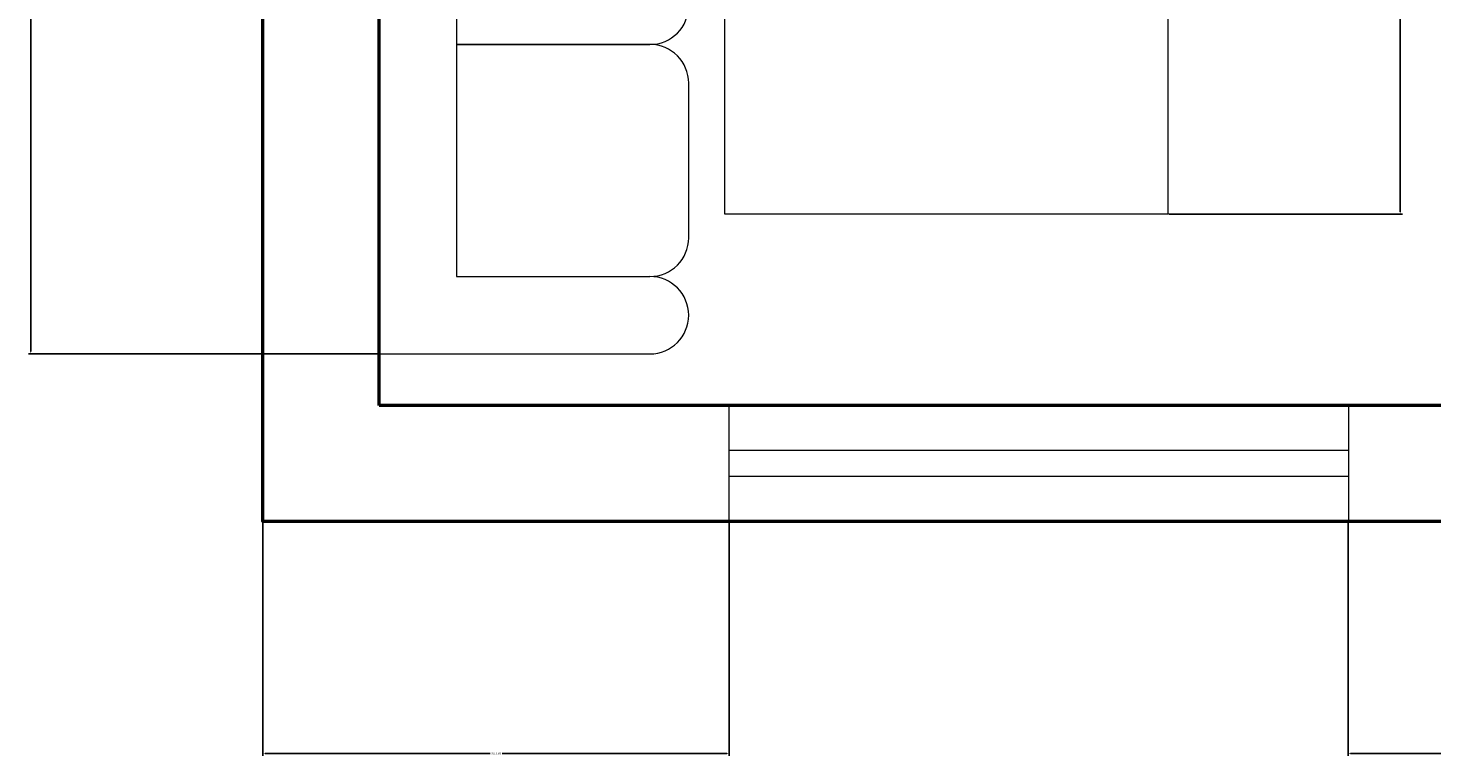
# Model space of a CAD drawing. Units: inches. Extents: x 2621 to 2849, y 2066 to 2463.
# Tile 1 of 28: x 2621 to 2729, y 2066 to 2123. Entities that reach past the tile are written whole.
import ezdxf

# ---------------------------------------------------------------- set-up
doc = ezdxf.new("R2010")
doc.units = ezdxf.units.IN
for name, color, linetype, lineweight in [('A-ANNO-DIMS', 2, 'Continuous', 18), ('A-FURN', 8, 'Continuous', 18), ('A-GLAZ', 4, 'Continuous', 18), ('A-WALL', 7, 'Continuous', 50)]:
    doc.layers.add(name, color=color, linetype=linetype, lineweight=lineweight)
doc.styles.get("Standard").update_dxf_attribs({"font": 'arial.ttf'})
doc.dimstyles.get("Standard").update_dxf_attribs({"dimtxt": 0.18, "dimasz": 0.18, "dimexe": 0.18, "dimexo": 0.0625, "dimgap": 0.09, "dimtad": 0, "dimtih": 1, "dimtoh": 1, "dimdec": 4, "dimzin": 0, "dimdsep": 46, "dimtxsty": 'Standard', "dimcen": 0.09, "dimadec": 0, "dimazin": 0, "dimtfac": 1, "dimtdec": 4, "dimtofl": 0, "dimtmove": 0, "dimatfit": 3, "dimfxl": 1, "dimtolj": 1, "dimtzin": 0, "dimarcsym": 0})

# ---------------------------------------------------------------- blocks, each defined once
blk = doc.blocks.new('WIN-48IN')
for p, q in [((0, 5.5), (48, 5.5)), ((0, 3.5), (48, 3.5))]:
    blk.add_line(p, q)
for points in [[(0, 0), (0, 9)], [(48, 9), (48, 0)]]:
    blk.add_lwpolyline(points)
blk = doc.blocks.new('*D40')
at = {"layer": 'A-ANNO-DIMS', "color": 0, "lineweight": -2, "transparency": 16777216}
for p, q in [((2638.87, 2084.31), (2638.87, 2066.19)), ((2675, 2084.31), (2675, 2066.19)), ((2639.05, 2066.37), (2656.47, 2066.37)), ((2674.82, 2066.37), (2657.4, 2066.37))]:
    blk.add_line(p, q, dxfattribs=at)
at = {"layer": 'A-ANNO-DIMS', "color": 0, "transparency": 16777216}
for points in [[(2639.05, 2066.4), (2639.05, 2066.34), (2638.87, 2066.37)], [(2674.82, 2066.4), (2674.82, 2066.34), (2675, 2066.37)]]:
    blk.add_solid(points, dxfattribs=at)
at = {"layer": 'Defpoints', "color": 0, "transparency": 16777216}
for p in [(2638.87, 2084.37), (2675, 2084.37), (2675, 2066.37)]:
    blk.add_point(p, dxfattribs=at)
at = {"layer": 'A-ANNO-DIMS', "color": 0, "transparency": 16777216, "insert": (2656.94, 2066.37), "char_height": 0.18, "attachment_point": 5}
blk.add_mtext('\\A1;36.135', dxfattribs=at)
blk = doc.blocks.new('*D41')
at = {"layer": 'A-ANNO-DIMS', "color": 0, "lineweight": -2, "transparency": 16777216}
for p, q in [((2723, 2084.31), (2723, 2066.19)), ((2761.87, 2084.31), (2761.87, 2066.19)), ((2723.18, 2066.37), (2741.97, 2066.37)), ((2761.69, 2066.37), (2742.9, 2066.37))]:
    blk.add_line(p, q, dxfattribs=at)
at = {"layer": 'A-ANNO-DIMS', "color": 0, "transparency": 16777216}
for points in [[(2723.18, 2066.4), (2723.18, 2066.34), (2723, 2066.37)], [(2761.69, 2066.4), (2761.69, 2066.34), (2761.87, 2066.37)]]:
    blk.add_solid(points, dxfattribs=at)
at = {"layer": 'Defpoints', "color": 0, "transparency": 16777216}
for p in [(2723, 2084.37), (2761.87, 2084.37), (2761.87, 2066.37)]:
    blk.add_point(p, dxfattribs=at)
at = {"layer": 'A-ANNO-DIMS', "color": 0, "transparency": 16777216, "insert": (2742.44, 2066.37), "char_height": 0.18, "attachment_point": 5}
blk.add_mtext('\\A1;38.865', dxfattribs=at)
blk = doc.blocks.new('*D62')
at = {"layer": 'A-ANNO-DIMS', "color": 0, "lineweight": -2, "transparency": 16777216}
for p, q in [((2647.81, 2199.37), (2620.69, 2199.37)), ((2620.87, 2199.19), (2620.87, 2148.56)), ((2620.87, 2097.55), (2620.87, 2148.19)), ((2647.81, 2097.37), (2620.69, 2097.37))]:
    blk.add_line(p, q, dxfattribs=at)
at = {"layer": 'A-ANNO-DIMS', "color": 0, "transparency": 16777216}
for points in [[(2620.84, 2199.19), (2620.9, 2199.19), (2620.87, 2199.37)], [(2620.84, 2097.55), (2620.9, 2097.55), (2620.87, 2097.37)]]:
    blk.add_solid(points, dxfattribs=at)
at = {"layer": 'Defpoints', "color": 0, "transparency": 16777216}
for p in [(2620.87, 2199.37), (2647.87, 2199.37), (2647.87, 2097.37)]:
    blk.add_point(p, dxfattribs=at)
at = {"layer": 'A-ANNO-DIMS', "color": 0, "transparency": 16777216, "insert": (2620.87, 2148.37), "char_height": 0.18, "attachment_point": 5}
blk.add_mtext('\\A1;102', dxfattribs=at)
blk = doc.blocks.new('*D64')
at = {"layer": 'A-ANNO-DIMS', "color": 0, "lineweight": -2, "transparency": 16777216}
for p, q in [((2709.08, 2168.2), (2727.2, 2168.2)), ((2727.02, 2168.02), (2727.02, 2138.39)), ((2727.02, 2108.38), (2727.02, 2138.02)), ((2709.08, 2108.2), (2727.2, 2108.2))]:
    blk.add_line(p, q, dxfattribs=at)
at = {"layer": 'A-ANNO-DIMS', "color": 0, "transparency": 16777216}
for points in [[(2726.99, 2168.02), (2727.05, 2168.02), (2727.02, 2168.2)], [(2726.99, 2108.38), (2727.05, 2108.38), (2727.02, 2108.2)]]:
    blk.add_solid(points, dxfattribs=at)
at = {"layer": 'Defpoints', "color": 0, "transparency": 16777216}
for p in [(2709.02, 2168.2), (2709.02, 2108.2), (2727.02, 2108.2)]:
    blk.add_point(p, dxfattribs=at)
at = {"layer": 'A-ANNO-DIMS', "color": 0, "transparency": 16777216, "insert": (2727.02, 2138.2), "char_height": 0.18, "attachment_point": 5}
blk.add_mtext('\\A1;60', dxfattribs=at)

msp = doc.modelspace()

# ---------------------------------------------------------------- linework, layer by layer
at = {"layer": 'A-FURN'}
for p, q in [((2647.8701, 2196.3746), (2647.8701, 2097.3746)), ((2653.8701, 2193.3746), (2653.8701, 2103.3746)), ((2653.8701, 2103.3746), (2668.8701, 2103.3746)), ((2671.8701, 2100.3746), (2671.8701, 2100.3746)), ((2647.8701, 2097.3746), (2668.8701, 2097.3746))]:
    msp.add_line(p, q, dxfattribs=at)
msp.add_lwpolyline([(2674.6703, 2168.2041), (2709.0205, 2168.2041), (2709.0205, 2108.2041), (2674.6703, 2108.2041)], close=True, dxfattribs=at)
for points in [[(2653.8701, 2121.3746), (2668.8701, 2121.3746, 0.41421356), (2671.8701, 2124.3746), (2671.8701, 2136.3746, 0.41421356), (2668.8701, 2139.3746), (2653.8701, 2139.3746)], [(2653.8701, 2103.3746), (2668.8701, 2103.3746, 0.41421356), (2671.8701, 2106.3746), (2671.8701, 2118.3746, 0.41421356), (2668.8701, 2121.3746), (2653.8701, 2121.3746)]]:
    msp.add_lwpolyline(points, format="xyb", close=True, dxfattribs=at)
for start, end in [(0, 90), (270, 0)]:
    msp.add_arc((2668.8701, 2100.3746), 3, start, end, dxfattribs=at)
at = {"layer": 'A-WALL'}
for p, q in [((2647.8701, 2093.3746), (2647.8701, 2199.3746)), ((2761.8701, 2093.3746), (2647.8701, 2093.3746))]:
    msp.add_line(p, q, dxfattribs=at)
msp.add_lwpolyline([(2761.8701, 2084.3746), (2638.8701, 2084.3746), (2638.8701, 2444.3746), (2830.8701, 2444.3746), (2830.8701, 2084.3746), (2797.8701, 2084.3746)], dxfattribs=at)

# ---------------------------------------------------------------- block references
at = {"layer": 'A-GLAZ', "rotation": 180}
msp.add_blockref('WIN-48IN', (2723.0048, 2093.3746), dxfattribs=at)

# ---------------------------------------------------------------- dimensions: what is measured, and where the dimension line sits
at = {"layer": 'A-ANNO-DIMS'}
for base, p1, p2, angle, picture, middle in [((2620.8666, 2199.3746), (2647.8701, 2097.3746), (2647.8701, 2199.3746), 90, '*D62', (2620.8666, 2148.3746)), ((2727.024, 2108.2041), (2709.0205, 2168.2041), (2709.0205, 2108.2041), 270, '*D64', (2727.024, 2138.2041))]:
    dim = msp.add_linear_dim(base=base, p1=p1, p2=p2, angle=angle, dimstyle='Standard', override={"dimdec": 0, "dimlfac": 1, "dimrnd": 0, "dimzin": 0, "dimdsep": 46, "dimlunit": 2}, dxfattribs=at)
    dim.commit()
    dim.dimension.update_dxf_attribs({"geometry": picture, "text_midpoint": middle})
for base, p1, p2, picture, middle in [((2675.0048, 2066.3711), (2638.8701, 2084.3746), (2675.0048, 2084.3746), '*D40', (2656.9374, 2066.3711)), ((2761.8701, 2066.3711), (2723.0048, 2084.3746), (2761.8701, 2084.3746), '*D41', (2742.4374, 2066.3711))]:
    dim = msp.add_linear_dim(base=base, p1=p1, p2=p2, dimstyle='Standard', override={"dimdec": 3, "dimlfac": 1, "dimrnd": 0, "dimzin": 0, "dimdsep": 46, "dimlunit": 2}, dxfattribs=at)
    dim.commit()
    dim.dimension.update_dxf_attribs({"geometry": picture, "text_midpoint": middle})

doc.saveas('drawing.dxf')
